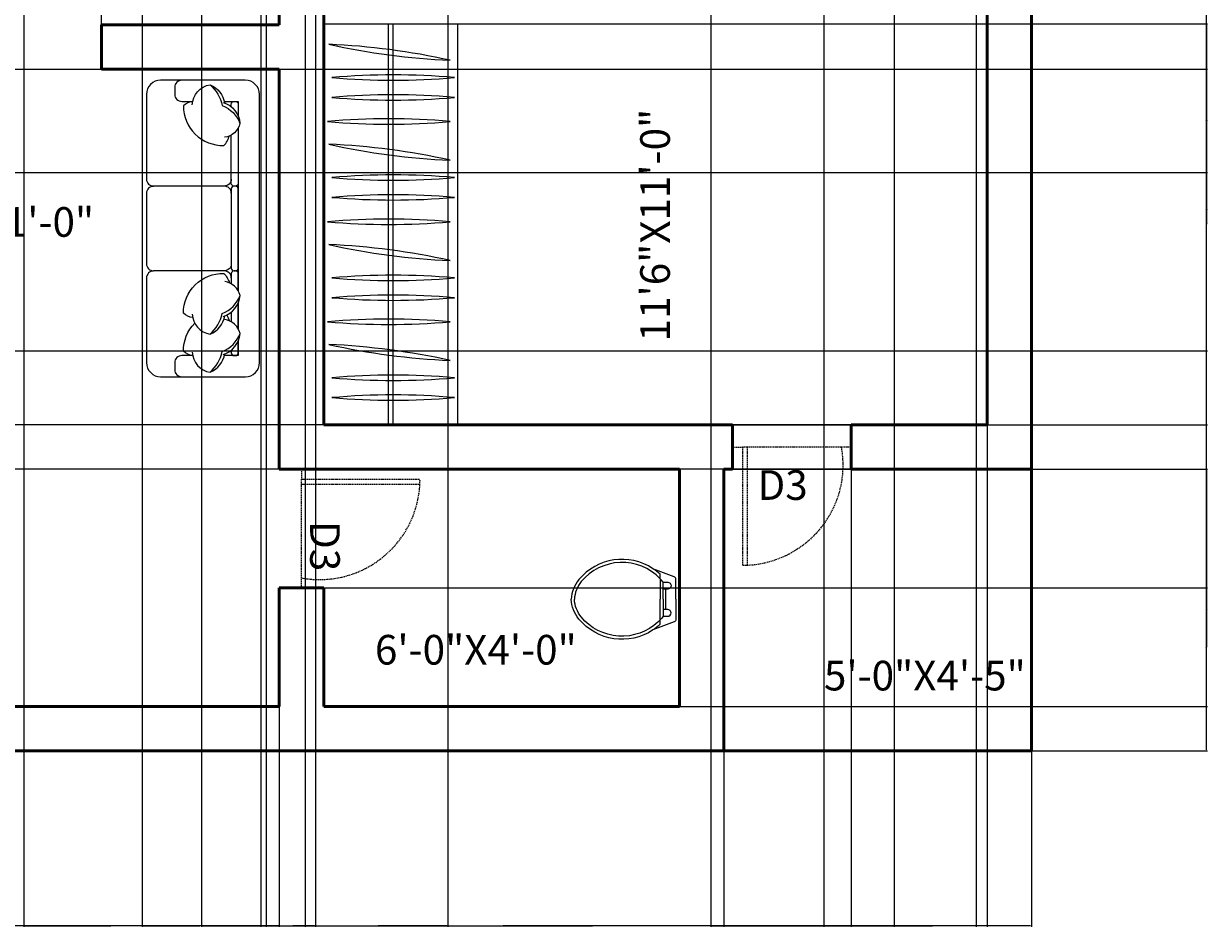
# Model space of a CAD drawing. Units: inches. Extents: x 3 to 576, y -689 to 51.
# Tile 9 of 21: x 336 to 576, y -689 to -506. Entities that reach past the tile are written whole.
import ezdxf

# ---------------------------------------------------------------- set-up
doc = ezdxf.new("R2010")
doc.units = ezdxf.units.IN
doc.header["$MEASUREMENT"] = 0
doc.linetypes.add('DASHED2', pattern=[0.375, 0.25, -0.125])
for name, color, linetype, lineweight in [('A-ANNO-DIMS', 2, 'Continuous', 18), ('A-ANNO-TEXT', 3, 'Continuous', 18), ('A-AREA-IDEN', 7, 'Continuous', 18), ('A-DOOR', 4, 'DASHED2', 25), ('A-FLOR-FIXT', 9, 'Continuous', 18), ('A-FURN', 8, 'Continuous', 18), ('A-WALL', 7, 'Continuous', 50)]:
    doc.layers.add(name, color=color, linetype=linetype, lineweight=lineweight)
doc.styles.get("Standard").update_dxf_attribs({"font": 'arial.ttf'})
doc.dimstyles.get("Standard").update_dxf_attribs({"dimtxt": 0.18, "dimasz": 0.18, "dimexe": 0.18, "dimexo": 0.0625, "dimgap": 0.09, "dimtad": 0, "dimtih": 1, "dimtoh": 1, "dimdec": 0, "dimzin": 0, "dimdsep": 46, "dimlunit": 3, "dimtxsty": 'Standard', "dimcen": 0.09, "dimadec": 0, "dimazin": 0, "dimtfac": 1, "dimtdec": 0, "dimtofl": 0, "dimtmove": 0, "dimatfit": 3, "dimfxl": 1, "dimtolj": 1, "dimtzin": 0, "dimarcsym": 0})

# ---------------------------------------------------------------- blocks, each defined once
blk = doc.blocks.new('SOFA-3SEAT')
at = {"ltscale": 0.03}
blk.add_lwpolyline([(2.86, 60.03, 0.414214), (0, 57.17), (0, 40.02, 0.414214), (1.43, 38.59, 0.414214), (0, 37.16), (0, 22.87, 0.414214), (1.43, 21.44, 0.414214), (0, 20.01), (0, 2.86, 0.414214), (2.86, 0), (20.01, 0, 0.414214), (22.87, 2.86), (22.87, 57.17, 0.414214), (20.01, 60.03)], format="xyb", close=True, dxfattribs=at)
for points in [[(7.15, 60.03, 0.414214), (5.72, 58.6), (5.72, 57.17, 0.414214), (7.15, 55.74), (9.36, 55.74)], [(9.27, 55.02, -0.356772), (12.88, 59.12, -0.249542), (15.84, 55.41, 9.61688)], [(12.88, 59.12, -0.14773), (15.33, 54.94, -0.213343), (18.93, 51.25, -0.178662)], [(9.36, 55.74, 0.165541), (7.47, 54.86, 0.425989), (15.66, 46.83, 0.121523), (16.79, 48.74, -7.115464)], [(15.53, 55.52, -0.306663), (18.93, 51.25, -0.30633), (15.82, 48.47, 0.872847)], [(17.15, 54.65), (17.15, 55.17, -0.414214), (17.72, 55.74), (18.01, 55.74, -0.414214), (18.58, 55.17)], [(18.58, 55.17), (18.58, 52.73, -0.414214)], [(18.58, 50.35), (18.58, 39.16, -0.414214), (18.01, 38.59), (17.72, 38.59, -0.414214), (17.15, 39.16), (17.15, 48.91, -0.414214)], [(17.15, 40.02, -0.414214), (15.72, 38.59), (1.43, 38.59, -0.414214)], [(17.15, 37.16, 0.414214), (15.72, 38.59)], [(17.15, 22.87, -0.414214), (15.72, 21.44)], [(17.15, 20.01, 0.414214), (15.72, 21.44), (1.43, 21.44, 0.414214)], [(9.36, 11.98, -0.165541), (7.47, 12.87, -0.425989), (15.66, 20.89, -0.121523), (16.79, 18.99, 7.115464)], [(15.53, 12.21, 0.306663), (18.93, 16.47, 0.30633), (15.82, 19.26, -0.872847)], [(18.58, 17.37), (18.58, 20.87, 0.414214), (18.01, 21.44), (17.72, 21.44, 0.414214), (17.15, 20.87), (17.15, 18.81, 0.414214)], [(12.88, 8.61, 0.14773), (15.33, 12.79, 0.213343), (18.93, 16.47, 0.178662)], [(18.58, 9.67), (18.58, 14.99, 0.414214)], [(9.27, 12.7, 0.356772), (12.88, 8.61, 0.249542), (15.84, 12.32, -9.61688)], [(16.23, 12.49, -0.071865), (16.79, 11.29, 7.115464)], [(17.15, 13.08), (17.15, 11.11, 0.414214)], [(9.36, 4.28, -0.165541), (7.47, 5.17, -0.200231), (9.77, 10.84, -0.121523)], [(15.53, 4.51, 0.306663), (18.93, 8.77, 0.30633), (15.82, 11.56, -0.872847)], [(12.88, 0.91, 0.14773), (15.33, 5.09, 0.213343), (18.93, 8.77, 0.178662)], [(18.58, 7.29), (18.58, 4.29), (15.77, 4.29, 0.414214)], [(18.58, 4.86), (18.58, 7.29, 0.414214)], [(9.27, 5, 0.356772), (12.88, 0.91, 0.249542), (15.84, 4.62, -9.61688)], [(17.15, 5.38), (17.15, 4.86, 0.414214), (17.72, 4.29), (18.01, 4.29, 0.414214), (18.58, 4.86)], [(9.36, 4.29), (7.15, 4.29, 0.414214), (5.72, 2.86), (5.72, 1.43, 0.414214), (7.15, 0)]]:
    blk.add_lwpolyline(points, format="xyb")
for points in [[(15.77, 55.74), (18.58, 55.74), (18.58, 52.73)], [(18.58, 50.35), (18.58, 17.37)], [(18.58, 14.99), (18.58, 9.67)]]:
    blk.add_lwpolyline(points)
blk.add_lwpolyline([(18.58, 22.01), (18.58, 38.02, 0.414214), (18.01, 38.59), (17.72, 38.59, 0.414214), (17.15, 38.02), (17.15, 22.01, 0.414214), (17.72, 21.44), (18.01, 21.44, 0.414214)], format="xyb", close=True)
blk = doc.blocks.new('WC-2')
for p, q in [((17.99, 12.27), (17.99, 13.16)), ((17.99, 12.27), (17.99, 8.1)), ((17.99, 3.93), (17.99, 8.1)), ((17.99, 3.04), (17.99, 3.93))]:
    blk.add_line(p, q)
for points in [[(16.53, 14.3, 0.383919), (1.53, 12.08, 0.163732), (0, 8.1, 0.359733)], [(17.99, 12.27, 0.448546), (2.02, 11.68, 0.162618), (0.63, 8.1, 0.470877)], [(17.99, 13.16, 0.040937), (16.53, 14.3, 0.163732)], [(21.19, 8.1), (21.19, 12.14, 0.31031), (20.85, 12.64), (16.53, 14.3, 0.209071)], [(18.62, 11.54, 0.022712), (17.99, 12.27, 0.162618)], [(18.62, 8.1), (18.62, 11.54, 0.476108)], [(18.62, 11.54), (19.51, 11.54, -1), (19.51, 10.18), (19.05, 10.18)], [(16.53, 1.89, -0.383919), (1.53, 4.11, -0.163732), (0, 8.1, -0.359733)], [(17.55, 3.5, -0.431639), (2.02, 4.52, -0.162618), (0.63, 8.1, -0.470877)], [(21.19, 8.1), (21.19, 4.05, -0.31031), (20.85, 3.55), (16.53, 1.89, -0.209071)], [(18.62, 8.1), (18.62, 4.66, -0.022712)], [(18.62, 4.66), (19.51, 4.66, 1), (19.51, 6.01), (19.05, 6.01)], [(17.99, 3.04, -0.040937), (16.53, 1.89, -0.163732)], [(17.99, 3.93, -0.014165), (17.55, 3.5, -0.162618)], [(18.62, 4.66, -0.022712), (17.99, 3.93, -0.162618)]]:
    blk.add_lwpolyline(points, format="xyb")
for points in [[(19.05, 10.18), (18.62, 10.18)], [(19.05, 10.18), (19.05, 6.01)], [(19.05, 6.01), (18.62, 6.01)]]:
    blk.add_lwpolyline(points)
blk = doc.blocks.new('DOOR-SWING-750')
for p, q in [((24, 24), (24, 22)), ((24, 22), (24, 2)), ((24, 2), (0, 2)), ((24, 0), (24, 2))]:
    blk.add_line(p, q)
blk.add_arc((20.33, 2), 20.33, 79.6111, 180)
blk = doc.blocks.new('*D39')
at = {"layer": 'A-ANNO-DIMS', "color": 0, "lineweight": -2, "transparency": 16777216}
for p, q in [((540.36, 15.69), (575.92, 15.69)), ((575.74, 15.51), (575.74, -318.63)), ((575.74, -653.13), (575.74, -318.99)), ((540.36, -653.31), (575.92, -653.31))]:
    blk.add_line(p, q, dxfattribs=at)
at = {"layer": 'A-ANNO-DIMS', "color": 0, "transparency": 16777216}
for points in [[(575.71, 15.51), (575.77, 15.51), (575.74, 15.69)], [(575.71, -653.13), (575.77, -653.13), (575.74, -653.31)]]:
    blk.add_solid(points, dxfattribs=at)
at = {"layer": 'Defpoints', "color": 0, "transparency": 16777216}
for p in [(540.29, 15.69), (540.29, -653.31), (575.74, -653.31)]:
    blk.add_point(p, dxfattribs=at)
at = {"layer": 'A-ANNO-DIMS', "color": 0, "transparency": 16777216, "insert": (575.74, -318.81), "char_height": 0.18, "attachment_point": 5}
blk.add_mtext('\\A1;55\'-9"', dxfattribs=at)
blk = doc.blocks.new('*D50')
at = {"layer": 'A-ANNO-DIMS', "color": 0, "lineweight": -2, "transparency": 16777216}
for p, q in [((388.02, -644.37), (388.02, -688.94)), ((102.29, -653.37), (102.29, -688.94)), ((102.47, -688.76), (244.55, -688.76)), ((387.84, -688.76), (245.77, -688.76))]:
    blk.add_line(p, q, dxfattribs=at)
at = {"layer": 'A-ANNO-DIMS', "color": 0, "transparency": 16777216}
for points in [[(102.47, -688.73), (102.47, -688.79), (102.29, -688.76)], [(387.84, -688.73), (387.84, -688.79), (388.02, -688.76)]]:
    blk.add_solid(points, dxfattribs=at)
at = {"layer": 'Defpoints', "color": 0, "transparency": 16777216}
for p in [(388.02, -644.31), (102.29, -653.31), (388.02, -688.76)]:
    blk.add_point(p, dxfattribs=at)
at = {"layer": 'A-ANNO-DIMS', "color": 0, "transparency": 16777216, "insert": (245.16, -688.76), "char_height": 0.18, "attachment_point": 5}
blk.add_mtext('\\A1;23\'-9 1/2"', dxfattribs=at)
blk = doc.blocks.new('*D51')
at = {"layer": 'A-ANNO-DIMS', "color": 0, "lineweight": -2, "transparency": 16777216}
for p, q in [((388.02, -644.37), (388.02, -688.94)), ((478.02, -653.37), (478.02, -688.94)), ((388.2, -688.76), (432.69, -688.76)), ((477.84, -688.76), (433.35, -688.76))]:
    blk.add_line(p, q, dxfattribs=at)
at = {"layer": 'A-ANNO-DIMS', "color": 0, "transparency": 16777216}
for points in [[(388.2, -688.73), (388.2, -688.79), (388.02, -688.76)], [(477.84, -688.73), (477.84, -688.79), (478.02, -688.76)]]:
    blk.add_solid(points, dxfattribs=at)
at = {"layer": 'Defpoints', "color": 0, "transparency": 16777216}
for p in [(388.02, -644.31), (478.02, -653.31), (478.02, -688.76)]:
    blk.add_point(p, dxfattribs=at)
at = {"layer": 'A-ANNO-DIMS', "color": 0, "transparency": 16777216, "insert": (433.02, -688.76), "char_height": 0.18, "attachment_point": 5}
blk.add_mtext('\\A1;7\'-6"', dxfattribs=at)
blk = doc.blocks.new('*D52')
at = {"layer": 'A-ANNO-DIMS', "color": 0, "lineweight": -2, "transparency": 16777216}
for p, q in [((478.02, -653.37), (478.02, -688.94)), ((540.29, -653.37), (540.29, -688.94)), ((478.2, -688.76), (508.62, -688.76)), ((540.11, -688.76), (509.7, -688.76))]:
    blk.add_line(p, q, dxfattribs=at)
at = {"layer": 'A-ANNO-DIMS', "color": 0, "transparency": 16777216}
for points in [[(478.2, -688.73), (478.2, -688.79), (478.02, -688.76)], [(540.11, -688.73), (540.11, -688.79), (540.29, -688.76)]]:
    blk.add_solid(points, dxfattribs=at)
at = {"layer": 'Defpoints', "color": 0, "transparency": 16777216}
for p in [(478.02, -653.31), (540.29, -653.31), (540.29, -688.76)]:
    blk.add_point(p, dxfattribs=at)
at = {"layer": 'A-ANNO-DIMS', "color": 0, "transparency": 16777216, "insert": (509.16, -688.76), "char_height": 0.18, "attachment_point": 5}
blk.add_mtext('\\A1;5\'-2 1/2"', dxfattribs=at)
blk = doc.blocks.new('*D73')
at = {"layer": 'A-ANNO-DIMS', "color": 0, "lineweight": -2, "transparency": 16777216}
for p, q in [((531.23, -449.31), (2.66, -449.31)), ((2.84, -449.49), (2.84, -518.13)), ((2.84, -587.13), (2.84, -518.49)), ((531.23, -587.31), (2.66, -587.31))]:
    blk.add_line(p, q, dxfattribs=at)
at = {"layer": 'A-ANNO-DIMS', "color": 0, "transparency": 16777216}
for points in [[(2.81, -449.49), (2.87, -449.49), (2.84, -449.31)], [(2.81, -587.13), (2.87, -587.13), (2.84, -587.31)]]:
    blk.add_solid(points, dxfattribs=at)
at = {"layer": 'Defpoints', "color": 0, "transparency": 16777216}
for p in [(531.29, -449.31), (2.84, -587.31), (531.29, -587.31)]:
    blk.add_point(p, dxfattribs=at)
at = {"layer": 'A-ANNO-DIMS', "color": 0, "transparency": 16777216, "insert": (2.84, -518.31), "char_height": 0.18, "attachment_point": 5}
blk.add_mtext('\\A1;11\'-6"', dxfattribs=at)
blk = doc.blocks.new('*D74')
at = {"layer": 'A-ANNO-DIMS', "color": 0, "lineweight": -2, "transparency": 16777216}
for p, q in [((531.23, -587.31), (2.66, -587.31)), ((2.84, -587.49), (2.84, -591.63)), ((2.84, -596.13), (2.84, -591.99)), ((540.23, -596.31), (2.66, -596.31))]:
    blk.add_line(p, q, dxfattribs=at)
at = {"layer": 'A-ANNO-DIMS', "color": 0, "transparency": 16777216}
for points in [[(2.81, -587.49), (2.87, -587.49), (2.84, -587.31)], [(2.81, -596.13), (2.87, -596.13), (2.84, -596.31)]]:
    blk.add_solid(points, dxfattribs=at)
at = {"layer": 'Defpoints', "color": 0, "transparency": 16777216}
for p in [(531.29, -587.31), (2.84, -596.31), (540.29, -596.31)]:
    blk.add_point(p, dxfattribs=at)
at = {"layer": 'A-ANNO-DIMS', "color": 0, "transparency": 16777216, "insert": (2.84, -591.81), "char_height": 0.18, "attachment_point": 5}
blk.add_mtext('\\A1;0\'-9"', dxfattribs=at)
blk = doc.blocks.new('*D75')
at = {"layer": 'A-ANNO-DIMS', "color": 0, "lineweight": -2, "transparency": 16777216}
for p, q in [((478.08, -596.31), (575.92, -596.31)), ((575.74, -596.49), (575.74, -624.63)), ((575.74, -653.13), (575.74, -624.99)), ((478.08, -653.31), (575.92, -653.31))]:
    blk.add_line(p, q, dxfattribs=at)
at = {"layer": 'A-ANNO-DIMS', "color": 0, "transparency": 16777216}
for points in [[(575.71, -596.49), (575.77, -596.49), (575.74, -596.31)], [(575.71, -653.13), (575.77, -653.13), (575.74, -653.31)]]:
    blk.add_solid(points, dxfattribs=at)
at = {"layer": 'Defpoints', "color": 0, "transparency": 16777216}
for p in [(478.02, -596.31), (478.02, -653.31), (575.74, -653.31)]:
    blk.add_point(p, dxfattribs=at)
at = {"layer": 'A-ANNO-DIMS', "color": 0, "transparency": 16777216, "insert": (575.74, -624.81), "char_height": 0.18, "attachment_point": 5}
blk.add_mtext('\\A1;4\'-9"', dxfattribs=at)
blk = doc.blocks.new('*D76')
at = {"layer": 'A-ANNO-DIMS', "color": 0, "lineweight": -2, "transparency": 16777216}
for p, q in [((372.29, -263.37), (372.29, -688.94)), ((336.29, -296.37), (336.29, -688.94)), ((336.47, -688.76), (353.96, -688.76)), ((372.11, -688.76), (354.62, -688.76))]:
    blk.add_line(p, q, dxfattribs=at)
at = {"layer": 'A-ANNO-DIMS', "color": 0, "transparency": 16777216}
for points in [[(336.47, -688.73), (336.47, -688.79), (336.29, -688.76)], [(372.11, -688.73), (372.11, -688.79), (372.29, -688.76)]]:
    blk.add_solid(points, dxfattribs=at)
at = {"layer": 'Defpoints', "color": 0, "transparency": 16777216}
for p in [(372.29, -263.31), (336.29, -296.31), (372.29, -688.76)]:
    blk.add_point(p, dxfattribs=at)
at = {"layer": 'A-ANNO-DIMS', "color": 0, "transparency": 16777216, "insert": (354.29, -688.76), "char_height": 0.18, "attachment_point": 5}
blk.add_mtext('\\A1;3\'-0"', dxfattribs=at)
blk = doc.blocks.new('*D77')
at = {"layer": 'A-ANNO-DIMS', "color": 0, "lineweight": -2, "transparency": 16777216}
for p, q in [((372.29, -263.37), (372.29, -688.94)), ((531.29, -263.37), (531.29, -688.94)), ((372.47, -688.76), (451.4, -688.76)), ((531.11, -688.76), (452.18, -688.76))]:
    blk.add_line(p, q, dxfattribs=at)
at = {"layer": 'A-ANNO-DIMS', "color": 0, "transparency": 16777216}
for points in [[(372.47, -688.73), (372.47, -688.79), (372.29, -688.76)], [(531.11, -688.73), (531.11, -688.79), (531.29, -688.76)]]:
    blk.add_solid(points, dxfattribs=at)
at = {"layer": 'Defpoints', "color": 0, "transparency": 16777216}
for p in [(372.29, -263.31), (531.29, -263.31), (531.29, -688.76)]:
    blk.add_point(p, dxfattribs=at)
at = {"layer": 'A-ANNO-DIMS', "color": 0, "transparency": 16777216, "insert": (451.79, -688.76), "char_height": 0.18, "attachment_point": 5}
blk.add_mtext('\\A1;13\'-3"', dxfattribs=at)
blk = doc.blocks.new('*D80')
at = {"layer": 'A-ANNO-DIMS', "color": 0, "lineweight": -2, "transparency": 16777216}
for p, q in [((372.29, -359.37), (372.29, -688.94)), ((385.37, -359.37), (385.37, -688.94)), ((372.47, -688.76), (378.51, -688.76)), ((385.19, -688.76), (379.15, -688.76))]:
    blk.add_line(p, q, dxfattribs=at)
at = {"layer": 'A-ANNO-DIMS', "color": 0, "transparency": 16777216}
for points in [[(372.47, -688.73), (372.47, -688.79), (372.29, -688.76)], [(385.19, -688.73), (385.19, -688.79), (385.37, -688.76)]]:
    blk.add_solid(points, dxfattribs=at)
at = {"layer": 'Defpoints', "color": 0, "transparency": 16777216}
for p in [(372.29, -359.31), (385.37, -359.31), (385.37, -688.76)]:
    blk.add_point(p, dxfattribs=at)
at = {"layer": 'A-ANNO-DIMS', "color": 0, "transparency": 16777216, "insert": (378.83, -688.76), "char_height": 0.18, "attachment_point": 5}
blk.add_mtext('\\A1;1\'-1"', dxfattribs=at)
blk = doc.blocks.new('*D81')
at = {"layer": 'A-ANNO-DIMS', "color": 0, "lineweight": -2, "transparency": 16777216}
for p, q in [((385.37, -359.37), (385.37, -688.94)), ((395.37, -359.37), (395.37, -688.94)), ((385.55, -688.76), (389.97, -688.76)), ((395.19, -688.76), (390.76, -688.76))]:
    blk.add_line(p, q, dxfattribs=at)
at = {"layer": 'A-ANNO-DIMS', "color": 0, "transparency": 16777216}
for points in [[(385.55, -688.73), (385.55, -688.79), (385.37, -688.76)], [(395.19, -688.73), (395.19, -688.79), (395.37, -688.76)]]:
    blk.add_solid(points, dxfattribs=at)
at = {"layer": 'Defpoints', "color": 0, "transparency": 16777216}
for p in [(385.37, -359.31), (395.37, -359.31), (395.37, -688.76)]:
    blk.add_point(p, dxfattribs=at)
at = {"layer": 'A-ANNO-DIMS', "color": 0, "transparency": 16777216, "insert": (390.37, -688.76), "char_height": 0.18, "attachment_point": 5}
blk.add_mtext('\\A1;0\'-10"', dxfattribs=at)
blk = doc.blocks.new('*D82')
at = {"layer": 'A-ANNO-DIMS', "color": 0, "lineweight": -2, "transparency": 16777216}
for p, q in [((395.37, -359.37), (395.37, -688.94)), ((475.37, -359.37), (475.37, -688.94)), ((395.55, -688.76), (435.04, -688.76)), ((475.19, -688.76), (435.7, -688.76))]:
    blk.add_line(p, q, dxfattribs=at)
at = {"layer": 'A-ANNO-DIMS', "color": 0, "transparency": 16777216}
for points in [[(395.55, -688.73), (395.55, -688.79), (395.37, -688.76)], [(475.19, -688.73), (475.19, -688.79), (475.37, -688.76)]]:
    blk.add_solid(points, dxfattribs=at)
at = {"layer": 'Defpoints', "color": 0, "transparency": 16777216}
for p in [(395.37, -359.31), (475.37, -359.31), (475.37, -688.76)]:
    blk.add_point(p, dxfattribs=at)
at = {"layer": 'A-ANNO-DIMS', "color": 0, "transparency": 16777216, "insert": (435.37, -688.76), "char_height": 0.18, "attachment_point": 5}
blk.add_mtext('\\A1;6\'-8"', dxfattribs=at)
blk = doc.blocks.new('*D83')
at = {"layer": 'A-ANNO-DIMS', "color": 0, "lineweight": -2, "transparency": 16777216}
for p, q in [((475.37, -359.37), (475.37, -688.94)), ((531.29, -359.37), (531.29, -688.94)), ((475.55, -688.76), (503, -688.76)), ((531.11, -688.76), (503.66, -688.76))]:
    blk.add_line(p, q, dxfattribs=at)
at = {"layer": 'A-ANNO-DIMS', "color": 0, "transparency": 16777216}
for points in [[(475.55, -688.73), (475.55, -688.79), (475.37, -688.76)], [(531.11, -688.73), (531.11, -688.79), (531.29, -688.76)]]:
    blk.add_solid(points, dxfattribs=at)
at = {"layer": 'Defpoints', "color": 0, "transparency": 16777216}
for p in [(475.37, -359.31), (531.29, -359.31), (531.29, -688.76)]:
    blk.add_point(p, dxfattribs=at)
at = {"layer": 'A-ANNO-DIMS', "color": 0, "transparency": 16777216, "insert": (503.33, -688.76), "char_height": 0.18, "attachment_point": 5}
blk.add_mtext('\\A1;4\'-8"', dxfattribs=at)
blk = doc.blocks.new('*D93')
at = {"layer": 'A-ANNO-DIMS', "color": 0, "lineweight": -2, "transparency": 16777216}
for p, q in [((174.14, -515.31), (575.92, -515.31)), ((575.74, -515.49), (575.74, -525.59)), ((575.74, -536.06), (575.74, -525.96)), ((174.14, -536.24), (575.92, -536.24))]:
    blk.add_line(p, q, dxfattribs=at)
at = {"layer": 'A-ANNO-DIMS', "color": 0, "transparency": 16777216}
for points in [[(575.71, -515.49), (575.77, -515.49), (575.74, -515.31)], [(575.71, -536.06), (575.77, -536.06), (575.74, -536.24)]]:
    blk.add_solid(points, dxfattribs=at)
at = {"layer": 'Defpoints', "color": 0, "transparency": 16777216}
for p in [(174.08, -515.31), (174.08, -536.24), (575.74, -536.24)]:
    blk.add_point(p, dxfattribs=at)
at = {"layer": 'A-ANNO-DIMS', "color": 0, "transparency": 16777216, "insert": (575.74, -525.77), "char_height": 0.18, "attachment_point": 5}
blk.add_mtext('\\A1;1\'-9"', dxfattribs=at)
blk = doc.blocks.new('*D94')
at = {"layer": 'A-ANNO-DIMS', "color": 0, "lineweight": -2, "transparency": 16777216}
for p, q in [((393.29, -136.9), (393.29, -688.94)), ((422.14, -136.9), (422.14, -688.94)), ((393.47, -688.76), (407.39, -688.76)), ((421.96, -688.76), (408.05, -688.76))]:
    blk.add_line(p, q, dxfattribs=at)
at = {"layer": 'A-ANNO-DIMS', "color": 0, "transparency": 16777216}
for points in [[(393.47, -688.73), (393.47, -688.79), (393.29, -688.76)], [(421.96, -688.73), (421.96, -688.79), (422.14, -688.76)]]:
    blk.add_solid(points, dxfattribs=at)
at = {"layer": 'Defpoints', "color": 0, "transparency": 16777216}
for p in [(393.29, -136.84), (422.14, -136.84), (422.14, -688.76)]:
    blk.add_point(p, dxfattribs=at)
at = {"layer": 'A-ANNO-DIMS', "color": 0, "transparency": 16777216, "insert": (407.72, -688.76), "char_height": 0.18, "attachment_point": 5}
blk.add_mtext('\\A1;2\'-5"', dxfattribs=at)
blk = doc.blocks.new('*D97')
at = {"layer": 'A-ANNO-DIMS', "color": 0, "lineweight": -2, "transparency": 16777216}
for p, q in [((424.15, -506.1), (575.92, -506.1)), ((575.74, -506.28), (575.74, -546.52)), ((575.74, -587.13), (575.74, -546.89)), ((424.15, -587.31), (575.92, -587.31))]:
    blk.add_line(p, q, dxfattribs=at)
at = {"layer": 'A-ANNO-DIMS', "color": 0, "transparency": 16777216}
for points in [[(575.71, -506.28), (575.77, -506.28), (575.74, -506.1)], [(575.71, -587.13), (575.77, -587.13), (575.74, -587.31)]]:
    blk.add_solid(points, dxfattribs=at)
at = {"layer": 'Defpoints', "color": 0, "transparency": 16777216}
for p in [(424.09, -506.1), (424.09, -587.31), (575.74, -587.31)]:
    blk.add_point(p, dxfattribs=at)
at = {"layer": 'A-ANNO-DIMS', "color": 0, "transparency": 16777216, "insert": (575.74, -546.71), "char_height": 0.18, "attachment_point": 5}
blk.add_mtext('\\A1;6\'-9"', dxfattribs=at)
blk = doc.blocks.new('*D103')
at = {"layer": 'A-ANNO-DIMS', "color": 0, "lineweight": -2, "transparency": 16777216}
for p, q in [((498.29, -50.37), (498.29, -688.94)), ((531.29, -50.37), (531.29, -688.94)), ((498.47, -688.76), (514.46, -688.76)), ((531.11, -688.76), (515.12, -688.76))]:
    blk.add_line(p, q, dxfattribs=at)
at = {"layer": 'A-ANNO-DIMS', "color": 0, "transparency": 16777216}
for points in [[(498.47, -688.73), (498.47, -688.79), (498.29, -688.76)], [(531.11, -688.73), (531.11, -688.79), (531.29, -688.76)]]:
    blk.add_solid(points, dxfattribs=at)
at = {"layer": 'Defpoints', "color": 0, "transparency": 16777216}
for p in [(498.29, -50.31), (531.29, -50.31), (531.29, -688.76)]:
    blk.add_point(p, dxfattribs=at)
at = {"layer": 'A-ANNO-DIMS', "color": 0, "transparency": 16777216, "insert": (514.79, -688.76), "char_height": 0.18, "attachment_point": 5}
blk.add_mtext('\\A1;2\'-9"', dxfattribs=at)
blk = doc.blocks.new('*D107')
at = {"layer": 'A-ANNO-DIMS', "color": 0, "lineweight": -2, "transparency": 16777216}
for p, q in [((111.36, -515.31), (575.92, -515.31)), ((575.74, -515.49), (575.74, -543.63)), ((575.74, -572.13), (575.74, -543.99)), ((111.36, -572.31), (575.92, -572.31))]:
    blk.add_line(p, q, dxfattribs=at)
at = {"layer": 'A-ANNO-DIMS', "color": 0, "transparency": 16777216}
for points in [[(575.71, -515.49), (575.77, -515.49), (575.74, -515.31)], [(575.71, -572.13), (575.77, -572.13), (575.74, -572.31)]]:
    blk.add_solid(points, dxfattribs=at)
at = {"layer": 'Defpoints', "color": 0, "transparency": 16777216}
for p in [(111.29, -515.31), (111.29, -572.31), (575.74, -572.31)]:
    blk.add_point(p, dxfattribs=at)
at = {"layer": 'A-ANNO-DIMS', "color": 0, "transparency": 16777216, "insert": (575.74, -543.81), "char_height": 0.18, "attachment_point": 5}
blk.add_mtext('\\A1;4\'-9"', dxfattribs=at)
blk = doc.blocks.new('*D112')
at = {"layer": 'A-ANNO-DIMS', "color": 0, "lineweight": -2, "transparency": 16777216}
for p, q in [((397.08, -620.31), (575.92, -620.31)), ((575.74, -620.49), (575.74, -632.13)), ((575.74, -644.13), (575.74, -632.49)), ((397.08, -644.31), (575.92, -644.31))]:
    blk.add_line(p, q, dxfattribs=at)
at = {"layer": 'A-ANNO-DIMS', "color": 0, "transparency": 16777216}
for points in [[(575.71, -620.49), (575.77, -620.49), (575.74, -620.31)], [(575.71, -644.13), (575.77, -644.13), (575.74, -644.31)]]:
    blk.add_solid(points, dxfattribs=at)
at = {"layer": 'Defpoints', "color": 0, "transparency": 16777216}
for p in [(397.02, -620.31), (397.02, -644.31), (575.74, -644.31)]:
    blk.add_point(p, dxfattribs=at)
at = {"layer": 'A-ANNO-DIMS', "color": 0, "transparency": 16777216, "insert": (575.74, -632.31), "char_height": 0.18, "attachment_point": 5}
blk.add_mtext('\\A1;2\'-0"', dxfattribs=at)
blk = doc.blocks.new('*D113')
at = {"layer": 'A-ANNO-DIMS', "color": 0, "lineweight": -2, "transparency": 16777216}
for p, q in [((531.29, -587.37), (531.29, -688.94)), ((503.77, -596.37), (503.77, -688.94)), ((503.95, -688.76), (516.99, -688.76)), ((531.11, -688.76), (518.07, -688.76))]:
    blk.add_line(p, q, dxfattribs=at)
at = {"layer": 'A-ANNO-DIMS', "color": 0, "transparency": 16777216}
for points in [[(503.95, -688.73), (503.95, -688.79), (503.77, -688.76)], [(531.11, -688.73), (531.11, -688.79), (531.29, -688.76)]]:
    blk.add_solid(points, dxfattribs=at)
at = {"layer": 'Defpoints', "color": 0, "transparency": 16777216}
for p in [(531.29, -587.31), (503.77, -596.31), (531.29, -688.76)]:
    blk.add_point(p, dxfattribs=at)
at = {"layer": 'A-ANNO-DIMS', "color": 0, "transparency": 16777216, "insert": (517.53, -688.76), "char_height": 0.18, "attachment_point": 5}
blk.add_mtext('\\A1;2\'-3 1/2"', dxfattribs=at)
blk = doc.blocks.new('*D116')
at = {"layer": 'A-ANNO-DIMS', "color": 0, "lineweight": -2, "transparency": 16777216}
for p, q in [((360.29, -134.37), (360.29, -688.94)), ((384.29, -134.37), (384.29, -688.94)), ((360.47, -688.76), (371.96, -688.76)), ((384.11, -688.76), (372.62, -688.76))]:
    blk.add_line(p, q, dxfattribs=at)
at = {"layer": 'A-ANNO-DIMS', "color": 0, "transparency": 16777216}
for points in [[(360.47, -688.73), (360.47, -688.79), (360.29, -688.76)], [(384.11, -688.73), (384.11, -688.79), (384.29, -688.76)]]:
    blk.add_solid(points, dxfattribs=at)
at = {"layer": 'Defpoints', "color": 0, "transparency": 16777216}
for p in [(360.29, -134.31), (384.29, -134.31), (384.29, -688.76)]:
    blk.add_point(p, dxfattribs=at)
at = {"layer": 'A-ANNO-DIMS', "color": 0, "transparency": 16777216, "insert": (372.29, -688.76), "char_height": 0.18, "attachment_point": 5}
blk.add_mtext('\\A1;2\'-0"', dxfattribs=at)
blk = doc.blocks.new('*D118')
at = {"layer": 'A-ANNO-DIMS', "color": 0, "lineweight": -2, "transparency": 16777216}
for p, q in [((352.02, -506.25), (352.02, 51.32)), ((352.2, 51.14), (369.69, 51.14)), ((387.84, 51.14), (370.35, 51.14)), ((388.02, -506.25), (388.02, 51.32))]:
    blk.add_line(p, q, dxfattribs=at)
at = {"layer": 'A-ANNO-DIMS', "color": 0, "transparency": 16777216}
for points in [[(352.2, 51.17), (352.2, 51.11), (352.02, 51.14)], [(387.84, 51.17), (387.84, 51.11), (388.02, 51.14)]]:
    blk.add_solid(points, dxfattribs=at)
at = {"layer": 'Defpoints', "color": 0, "transparency": 16777216}
for p in [(388.02, 51.14), (352.02, -506.31), (388.02, -506.31)]:
    blk.add_point(p, dxfattribs=at)
at = {"layer": 'A-ANNO-DIMS', "color": 0, "transparency": 16777216, "insert": (370.02, 51.14), "char_height": 0.18, "attachment_point": 5}
blk.add_mtext('\\A1;3\'-0"', dxfattribs=at)
blk = doc.blocks.new('*D126')
at = {"layer": 'A-ANNO-DIMS', "color": 0, "lineweight": -2, "transparency": 16777216}
for p, q in [((512.51, -386.37), (512.51, -688.94)), ((529.12, -391.8), (529.12, -688.94)), ((512.69, -688.76), (520.28, -688.76)), ((528.94, -688.76), (521.35, -688.76))]:
    blk.add_line(p, q, dxfattribs=at)
at = {"layer": 'A-ANNO-DIMS', "color": 0, "transparency": 16777216}
for points in [[(512.69, -688.73), (512.69, -688.79), (512.51, -688.76)], [(528.94, -688.73), (528.94, -688.79), (529.12, -688.76)]]:
    blk.add_solid(points, dxfattribs=at)
at = {"layer": 'Defpoints', "color": 0, "transparency": 16777216}
for p in [(512.51, -386.31), (529.12, -391.74), (529.12, -688.76)]:
    blk.add_point(p, dxfattribs=at)
at = {"layer": 'A-ANNO-DIMS', "color": 0, "transparency": 16777216, "insert": (520.82, -688.76), "char_height": 0.18, "attachment_point": 5}
blk.add_mtext('\\A1;1\'-4 1/2"', dxfattribs=at)

msp = doc.modelspace()

# ---------------------------------------------------------------- linework, layer by layer
at = {"layer": 'A-DOOR'}
for p, q in [((482.77, -591.81), (482.77, -615.81)), ((392.52, -599.31), (416.52, -599.31))]:
    msp.add_line(p, q, dxfattribs=at)
at = {"layer": 'A-FURN'}
for p, q in [((397.02, -506.1), (397.02, -587.31)), ((397.02, -506.1), (424.09, -506.1)), ((410.1, -506.1), (410.1, -587.31)), ((411.01, -506.1), (411.01, -587.31)), ((424.09, -506.1), (424.09, -587.31)), ((397.02, -587.31), (424.09, -587.31))]:
    msp.add_line(p, q, dxfattribs=at)
for centre, start, end in [((428.84, -371.22), 257.508, 267.5023), ((391.83, -652.57), 77.508, 87.5023), ((411.1, -658.91), 85.0028, 94.9972), ((411.1, -375.13), 265.0028, 274.9972), ((411.1, -662.92), 85.0028, 94.9972), ((411.1, -379.14), 265.0028, 274.9972), ((410.22, -667.79), 85.0028, 94.9972), ((410.22, -384.02), 265.0028, 274.9972), ((428.84, -391.45), 257.508, 267.5023), ((391.83, -672.8), 77.508, 87.5023), ((411.1, -679.14), 85.0028, 94.9972), ((411.1, -395.36), 265.0028, 274.9972), ((411.1, -683.15), 85.0028, 94.9972), ((411.1, -399.37), 265.0028, 274.9972), ((410.22, -688.1), 85.0028, 94.9972), ((410.22, -404.32), 265.0028, 274.9972), ((391.83, -693.11), 77.508, 87.5023), ((428.84, -411.76), 257.508, 267.5023), ((411.1, -699.45), 85.0028, 94.9972), ((411.1, -415.67), 265.0028, 274.9972), ((411.1, -703.46), 85.0028, 94.9972), ((411.1, -419.68), 265.0028, 274.9972), ((410.22, -708.33), 85.0028, 94.9972), ((410.22, -424.56), 265.0028, 274.9972), ((391.83, -713.34), 77.508, 87.5023), ((428.84, -431.99), 257.508, 267.5023), ((411.1, -719.68), 85.0028, 94.9972), ((411.1, -435.9), 265.0028, 274.9972), ((411.1, -723.69), 85.0028, 94.9972), ((411.1, -439.91), 265.0028, 274.9972)]:
    msp.add_arc(centre, 142.43, start, end, dxfattribs=at)
at = {"layer": 'A-WALL'}
for p, q in [((540.29, 15.69), (540.29, -653.31)), ((531.29, -449.31), (531.29, -587.31)), ((388.02, -485.31), (388.02, -506.31)), ((397.02, -485.31), (397.02, -587.31)), ((352.02, -506.31), (352.02, -515.31)), ((352.02, -506.31), (388.02, -506.31)), ((352.02, -515.31), (388.02, -515.31)), ((388.02, -515.31), (388.02, -596.31)), ((397.02, -587.31), (479.77, -587.31)), ((479.77, -596.31), (479.77, -587.31)), ((503.77, -596.31), (503.77, -587.31)), ((503.77, -587.31), (531.29, -587.31)), ((388.02, -596.31), (469.02, -596.31)), ((469.02, -596.31), (469.02, -644.31)), ((478.02, -596.31), (478.02, -653.31)), ((478.02, -596.31), (479.77, -596.31)), ((503.77, -596.31), (540.29, -596.31)), ((397.02, -620.31), (388.02, -620.31)), ((388.02, -620.31), (388.02, -644.31)), ((397.02, -620.31), (397.02, -644.31)), ((264.29, -644.31), (388.02, -644.31)), ((397.02, -644.31), (469.02, -644.31)), ((38.29, -653.31), (540.29, -653.31))]:
    msp.add_line(p, q, dxfattribs=at)

# ---------------------------------------------------------------- block references
at = {"layer": 'A-DOOR', "extrusion": (0, 0, -1), "zscale": -1, "rotation": 90.00000000000007}
msp.add_blockref('DOOR-SWING-750', (-479.77, -615.81), dxfattribs=at)
at = {"layer": 'A-DOOR', "rotation": 180}
msp.add_blockref('DOOR-SWING-750', (416.52, -596.31), dxfattribs=at)
at = {"layer": 'A-FLOR-FIXT'}
msp.add_blockref('WC-2', (447.14, -630.73), dxfattribs=at)
at = {"layer": 'A-FURN', "rotation": 0.0124975635053893}
msp.add_blockref('SOFA-3SEAT', (361.16, -577.58), dxfattribs=at)

# ---------------------------------------------------------------- texts
at = {"layer": 'A-ANNO-TEXT', "insert": (484.82, -596.5), "char_height": 6, "attachment_point": 1}
msp.add_mtext('D3', dxfattribs=at)
at = {"layer": 'A-ANNO-TEXT', "insert": (400.28, -606.78), "char_height": 6, "attachment_point": 1, "rotation": 270}
msp.add_mtext('D3', dxfattribs=at)
at = {"layer": 'A-AREA-IDEN', "insert": (461.09, -570.42), "char_height": 6, "attachment_point": 1, "rotation": 90}
msp.add_mtext('11\'6"X11\'-0"', dxfattribs=at)
at = {"layer": 'A-AREA-IDEN', "char_height": 6, "attachment_point": 1}
for s, insert in [('10\'-0"X11\'-0"', (300.61, -543.24)), ('6\'-0"X4\'-0"', (407.39, -629.84)), ('5\'-0"X4\'-5"', (498.28, -635.08))]:
    msp.add_mtext(s, dxfattribs=dict(at, insert=insert))

# ---------------------------------------------------------------- dimensions: what is measured, and where the dimension line sits
at = {"layer": 'A-ANNO-DIMS'}
for base, p1, p2, picture, middle in [((388.02, 51.14), (352.02, -506.31), (388.02, -506.31), '*D118', (370.02, 51.14)), ((531.29, -688.76), (498.29, -50.31), (531.29, -50.31), '*D103', (514.79, -688.76)), ((384.29, -688.76), (360.29, -134.31), (384.29, -134.31), '*D116', (372.29, -688.76)), ((422.1383, -688.7597), (393.294, -136.8425), (422.1383, -136.8425), '*D94', (407.7162, -688.7597)), ((372.29, -688.76), (336.29, -296.31), (372.29, -263.31), '*D76', (354.29, -688.76)), ((531.29, -688.76), (372.29, -263.31), (531.29, -263.31), '*D77', (451.79, -688.76)), ((385.37, -688.76), (372.29, -359.31), (385.37, -359.31), '*D80', (378.83, -688.76)), ((395.37, -688.76), (385.37, -359.31), (395.37, -359.31), '*D81', (390.37, -688.76)), ((475.37, -688.76), (395.37, -359.31), (475.37, -359.31), '*D82', (435.37, -688.76)), ((531.29, -688.76), (475.37, -359.31), (531.29, -359.31), '*D83', (503.33, -688.76)), ((529.12, -688.76), (512.51, -386.31), (529.12, -391.74), '*D126', (520.82, -688.76)), ((531.29, -688.76), (503.77, -596.31), (531.29, -587.31), '*D113', (517.53, -688.76)), ((388.02, -688.76), (102.29, -653.31), (388.02, -644.31), '*D50', (245.16, -688.76)), ((478.02, -688.76), (388.02, -644.31), (478.02, -653.31), '*D51', (433.02, -688.76)), ((540.29, -688.76), (478.02, -653.31), (540.29, -653.31), '*D52', (509.16, -688.76))]:
    dim = msp.add_linear_dim(base=base, p1=p1, p2=p2, dimstyle='Standard', override={"dimdec": 1, "dimlfac": 1, "dimrnd": 0, "dimzin": 1, "dimdsep": 46, "dimlunit": 4, "dimfrac": 2}, dxfattribs=at)
    dim.commit()
    dim.dimension.update_dxf_attribs({"geometry": picture, "text_midpoint": middle})
for base, p1, p2, picture, middle in [((575.74, -653.31), (540.29, 15.69), (540.29, -653.31), '*D39', (575.74, -318.81)), ((2.84, -587.31), (531.29, -449.31), (531.29, -587.31), '*D73', (2.84, -518.31)), ((575.74, -587.31), (424.09, -506.1), (424.09, -587.31), '*D97', (575.74, -546.71)), ((575.74, -572.31), (111.29, -515.31), (111.29, -572.31), '*D107', (575.74, -543.81)), ((575.74, -536.24), (174.08, -515.31), (174.08, -536.24), '*D93', (575.74, -525.77)), ((2.84, -596.31), (531.29, -587.31), (540.29, -596.31), '*D74', (2.84, -591.81)), ((575.74, -653.31), (478.02, -596.31), (478.02, -653.31), '*D75', (575.74, -624.81)), ((575.74, -644.31), (397.02, -620.31), (397.02, -644.31), '*D112', (575.74, -632.31))]:
    dim = msp.add_linear_dim(base=base, p1=p1, p2=p2, angle=90, dimstyle='Standard', override={"dimdec": 1, "dimlfac": 1, "dimrnd": 0, "dimzin": 1, "dimdsep": 46, "dimlunit": 4, "dimfrac": 2}, dxfattribs=at)
    dim.commit()
    dim.dimension.update_dxf_attribs({"geometry": picture, "text_midpoint": middle})

doc.saveas('drawing.dxf')
